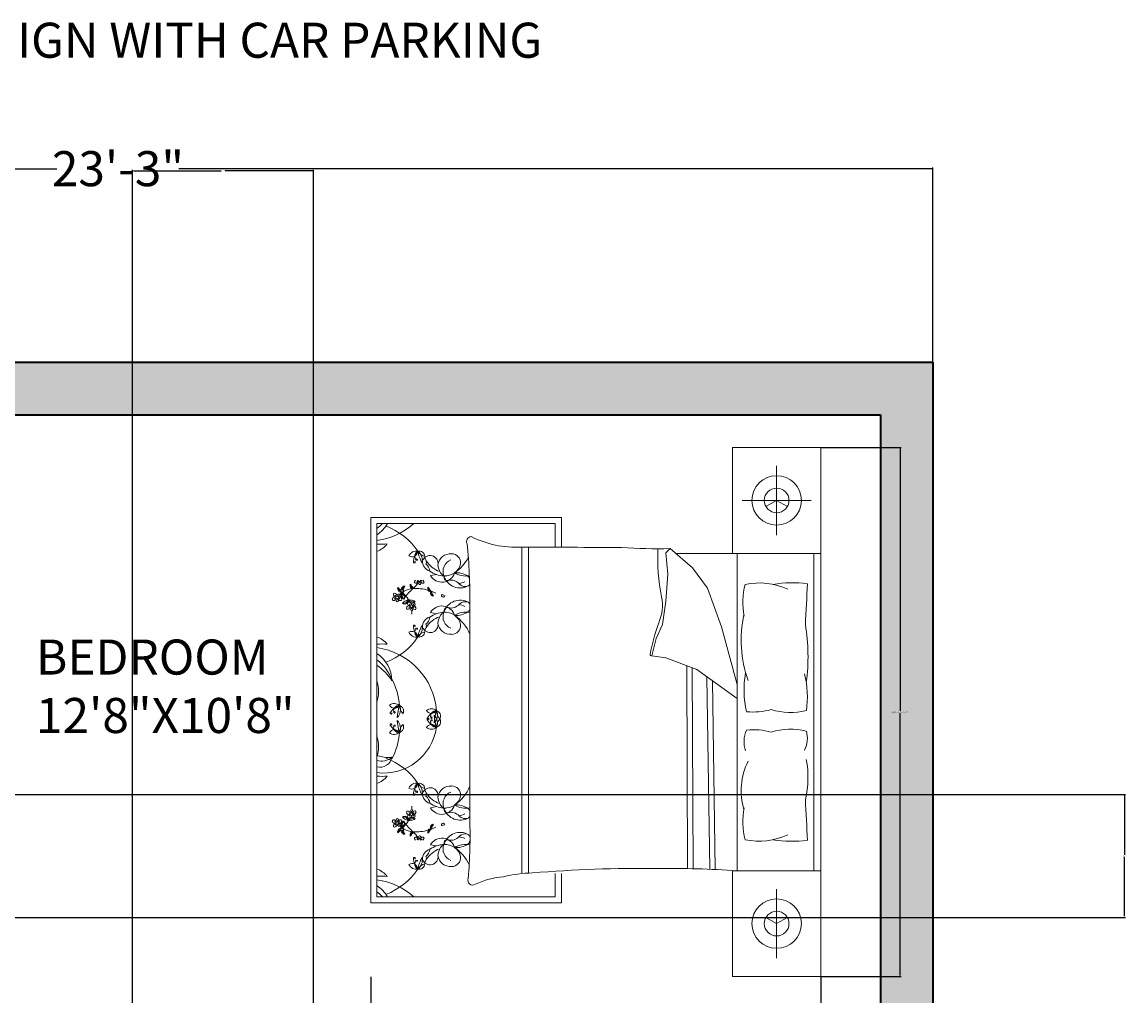
# Model space of a CAD drawing. Units: inches. Extents: x 37 to 706, y -568 to 110.
# Tile 24 of 24: x 517 to 706, y -57 to 110. Entities that reach past the tile are written whole.
import ezdxf

# ---------------------------------------------------------------- set-up
doc = ezdxf.new("R2010")
doc.units = ezdxf.units.IN
doc.header["$MEASUREMENT"] = 0
for name, color, linetype, lineweight in [('A-ANNO-DIMS', 2, 'Continuous', 18), ('A-ANNO-TEXT', 7, 'Continuous', 18), ('A-AREA-IDEN', 7, 'Continuous', 18), ('A-FURN', 8, 'Continuous', 13), ('A-WALL', 7, 'Continuous', 35), ('A-WALL-PATT', 252, 'Continuous', 13)]:
    doc.layers.add(name, color=color, linetype=linetype, lineweight=lineweight)
doc.styles.get("Standard").update_dxf_attribs({"font": 'arial.ttf'})
doc.dimstyles.get("Standard").update_dxf_attribs({"dimtxt": 0.18, "dimasz": 0.18, "dimexe": 0.18, "dimexo": 0.0625, "dimgap": 0.09, "dimtad": 0, "dimtih": 1, "dimtoh": 1, "dimdec": 0, "dimzin": 0, "dimdsep": 46, "dimlunit": 3, "dimtxsty": 'Standard', "dimcen": 0.09, "dimadec": 0, "dimazin": 0, "dimtfac": 1, "dimtdec": 0, "dimtofl": 0, "dimtmove": 0, "dimatfit": 3, "dimfxl": 1, "dimtolj": 1, "dimtzin": 0, "dimarcsym": 0})

# ---------------------------------------------------------------- blocks, each defined once
blk = doc.blocks.new('*D4')
at = {"layer": 'A-ANNO-DIMS', "color": 0, "lineweight": -2, "transparency": 16777216}
for p, q in [((393.96, 51.35), (393.96, 84.59)), ((394.14, 84.41), (523.01, 84.41)), ((672.78, 84.41), (543.91, 84.41)), ((672.96, 51.35), (672.96, 84.59))]:
    blk.add_line(p, q, dxfattribs=at)
at = {"layer": 'A-ANNO-DIMS', "color": 0, "transparency": 16777216}
for points in [[(394.14, 84.44), (394.14, 84.38), (393.96, 84.41)], [(672.78, 84.44), (672.78, 84.38), (672.96, 84.41)]]:
    blk.add_solid(points, dxfattribs=at)
at = {"layer": 'Defpoints', "color": 0, "transparency": 16777216}
for p in [(672.96, 84.41), (393.96, 51.29), (672.96, 51.29)]:
    blk.add_point(p, dxfattribs=at)
at = {"layer": 'A-ANNO-DIMS', "color": 0, "transparency": 16777216, "insert": (533.46, 84.41), "char_height": 6, "attachment_point": 5}
blk.add_mtext('\\A1;23\'-3"', dxfattribs=at)
blk = doc.blocks.new('BED-DOUBLE-WITH-NIGHTSTANDS')
for p, q in [((77.02, 90.57), (77.02, 0)), ((69.47, 75.59), (69.47, 87.43)), ((63.56, 81.51), (75.39, 81.51)), ((0, 78.61), (32.62, 78.61)), ((0, 12.59), (0, 78.61)), ((1.05, 77.56), (1.05, 13.64)), ((31.58, 77.56), (1.05, 77.56)), ((31.58, 73.49), (31.58, 77.56)), ((32.62, 78.61), (32.62, 73.49)), ((25.85, 17.62), (25.85, 73.5)), ((26.98, 17.7), (26.98, 73.5)), ((50.48, 72.53), (51.22, 73.26)), ((50.85, 68.86), (50.48, 72.53)), ((51.22, 73.26), (55.07, 69.96)), ((77.02, 72.45), (52.16, 72.45)), ((62.71, 72.45), (62.71, 18.11)), ((75.86, 18.11), (75.86, 72.45)), ((55.07, 69.96), (57.63, 66.48)), ((10.23, 68.64), (11.25, 68.84)), ((50.48, 64.28), (50.85, 68.86)), ((57.63, 66.48), (60.02, 59.87)), ((49.93, 60.24), (50.48, 64.28)), ((16.95, 26.9), (16.95, 63.67)), ((10.23, 62.31), (11.25, 62.11)), ((48.83, 57.86), (49.93, 60.24)), ((60.02, 59.87), (62.71, 50)), ((48.1, 54.92), (48.83, 57.86)), ((50.48, 54.55), (48.1, 54.92)), ((55.8, 52.54), (50.48, 54.55)), ((54.24, 18.43), (54.09, 53.18)), ((55.17, 18.44), (55.03, 52.83)), ((62.71, 47.57), (55.8, 52.54)), ((58.02, 18.39), (57.55, 51.28)), ((58.95, 18.36), (58.49, 50.6)), ((10.23, 28.89), (11.25, 29.09)), ((10.23, 22.56), (11.25, 22.36)), ((31.58, 13.64), (31.58, 17.63)), ((32.62, 17.61), (32.62, 12.59)), ((1.05, 13.64), (31.58, 13.64)), ((69.47, 14.97), (69.47, 3.14)), ((32.62, 12.59), (0, 12.59))]:
    blk.add_line(p, q)
for points in [[(61.93, 72.45), (61.93, 90.57), (77.02, 90.57)], [(69.47, 81.51), (67.64, 80.45)], [(69.47, 81.51), (71.3, 80.45)], [(77.02, 18.11), (61.93, 18.11), (61.93, 0), (77.02, 0)], [(69.47, 9.06), (67.64, 10.11)], [(69.47, 9.06), (71.3, 10.11)]]:
    blk.add_lwpolyline(points)
for points in [[(42.92, 73.45, 0.001242), (25.74, 73.5, -0.127202), (17.18, 75.31)], [(74.76, 67.25, 0.074897), (68.85, 67.14, -0.472817)], [(68.52, 45.71, 0.14099), (74.55, 45.53, 0.235245)], [(68.52, 41.84, -0.14099), (74.55, 42.02, -0.235245)], [(74.76, 23.32, -0.074897), (68.85, 23.42, 0.472817)], [(27.69, 17.73, 0.056112), (22.71, 17.07, 0.095341), (17.91, 15.8)]]:
    blk.add_lwpolyline(points, format="xyb")
for centre, radius in [((69.47, 81.51), 4.23), ((69.47, 81.51), 2.11), ((4.52, 64.91), 0.231), ((6.95, 63.41), 0.231), ((4.52, 26.28), 0.231), ((6.95, 27.79), 0.231), ((69.47, 9.06), 4.23), ((69.47, 9.06), 2.11)]:
    blk.add_circle(centre, radius)
for centre, radius, start, end in [((-3.2, 82.51), 7.18, 306.3036, 316.4814), ((-2.13, 80.43), 5.76, 303.4617, 330.1116), ((-0.54, 86.37), 11.83, 277.745, 311.8856), ((-1.71, 66.13), 11.83, 34.3865, 68.5908), ((-0.79, 77.21), 4.81, 292.5547, 318.9546), ((1.79, 90.38), 16.36, 267.4081, 273.6519), ((17.23, 74.48), 0.836, 93.98, 207.3412), ((-77.32, 64.75), 94.28, 359.3433, 5.6887), ((7.77, 71.53), 1.31, 77.7115, 159.0387), ((7.06, 72.84), 0.988, 238.4633, 358.2869), ((10.3, 70.85), 2.99, 138.8402, 177.9352), ((8.5, 71.96), 0.967, 117.6827, 223.7762), ((8.28, 71.86), 0.98, 2.9516, 103.728), ((16.12, 74.61), 8.27, 192.5173, 207.1824), ((6.95, 71.3), 1.87, 345.4653, 54.2343), ((9.77, 73.87), 2.02, 211.3827, 255.2969), ((10.16, 70.71), 1.36, 350.264, 160.8688), ((13.65, 70.21), 2.16, 84.9449, 172.8857), ((13.86, 70.84), 1.53, 354.4856, 91.0538), ((48.97, 156.3), 83.07, 265.8294, 271.553), ((83.29, 71.71), 34.18, 177.4519, 191.3392), ((7.46, 70.95), 0.147, 177.9352, 11.4834), ((7.53, 70.96), 0.0713, 11.4834, 127.9409), ((7.89, 71.38), 0.128, 223.7762, 159.7183), ((10.57, 71.04), 1.7, 175.969, 254.3045), ((8.69, 70.99), 0.833, 333.9755, 53.2681), ((8.31, 69.21), 1.81, 6.1662, 51.5825), ((13.15, 73.4), 4.28, 211.2614, 251.7045), ((14.13, 70.59), 2.63, 182.3591, 234.0401), ((14.47, 69.36), 2.1, 111.5819, 201.4221), ((12.73, 71.31), 2.72, 265.2933, 346.921), ((10.57, 74.83), 6.85, 303.6671, 333.2997), ((12.81, 73.44), 4.86, 236.2883, 266.5076), ((12.18, 69.76), 2.25, 209.9085, 343.1337), ((13.13, 68.34), 0.562, 167.3041, 285.1471), ((14.65, 65.65), 3.49, 122.7011, 126.3445), ((15.31, 69.41), 2.89, 199.2822, 299.1751), ((16.28, 72.32), 3.75, 238.8218, 279.1554), ((14.65, 65.65), 3.49, 55.785, 94.7304), ((15.95, 67.67), 1.09, 30.0293, 52.325), ((4.85, 66.4), 0.258, 124.3538, 214.3923), ((5.23, 66.36), 0.6, 190.3057, 287.1958), ((5.41, 66.58), 0.697, 176.9701, 248.2913), ((10.38, 70.25), 6.74, 212.6784, 216.3746), ((5.17, 66.41), 0.267, 216.3746, 291.7548), ((5.81, 66.23), 0.6, 122.8155, 187.3992), ((5.34, 65.98), 0.201, 289.3605, 111.7548), ((6.07, 66.15), 0.697, 109.4799, 177.6828), ((5.7, 66.59), 0.258, 56.8636, 146.9021), ((5.83, 66.31), 0.267, 148.8844, 224.2646), ((11.37, 62.96), 6.74, 145.1882, 148.8844), ((7.53, 62.67), 3.76, 94.756, 119.2041), ((15.54, 57.26), 12.37, 132.2412, 142.1744), ((9.29, 67.11), 2.55, 178.3264, 187.1302), ((6.53, 66.75), 0.476, 11.3256, 64.4621), ((8.15, 67.44), 1.43, 190.2588, 210.656), ((7.19, 66.85), 0.435, 188.3432, 274.2869), ((7.57, 67.09), 0.759, 210.656, 242.6341), ((8.14, 67.75), 1.46, 218.2101, 226.3071), ((7.07, 66.52), 0.185, 325.7657, 67.4417), ((1.34, 72.69), 8.6, 313.1541, 322.0459), ((7.72, 58.94), 7.5, 73.5842, 93.8277), ((7.66, 67.53), 0.177, 142.4737, 265.053), ((7.89, 67.56), 0.381, 127.7621, 169.0403), ((7.69, 67.89), 0.536, 265.053, 338.3618), ((8.4, 67.15), 0.7, 113.4276, 137.6104), ((8.32, 67.88), 0.231, 183.2768, 356.7232), ((8.49, 67.46), 0.377, 139.7889, 227.6792), ((8.37, 67.33), 0.199, 227.6792, 350.3487), ((7.6, 67.46), 0.755, 353.0852, 15.7171), ((8.1, 67.37), 0.477, 350.3487, 43.6538), ((8.98, 67.87), 0.555, 198.7263, 262.5032), ((8.54, 67.61), 0.22, 1.1081, 91.8675), ((8.68, 67.56), 0.385, 11.5637, 52.6358), ((8.95, 67.49), 0.178, 255.2356, 54.9248), ((12.34, 66.57), 2.55, 178.3264, 187.1302), ((9.58, 66.21), 0.476, 11.3256, 64.4621), ((11.19, 66.9), 1.43, 190.2588, 210.656), ((10.23, 66.31), 0.435, 188.3432, 274.2869), ((10.61, 66.55), 0.759, 210.656, 242.6341), ((11.19, 67.21), 1.46, 218.2101, 226.3071), ((10.11, 65.98), 0.185, 325.7657, 67.4417), ((13.76, 66), 1.86, 41.5653, 105.1471), ((14.78, 69.85), 2.6, 277.436, 299.9149), ((16.16, 68.13), 1.36, 221.5653, 293.8354), ((15.95, 67.67), 1.09, 314.4517, 333.558), ((75.82, 64.02), 12.14, 165.1039, 191.0369), ((66.47, 55.71), 11.67, 65.1316, 101.7583), ((936.66, 17.33), 863.34, 176.68521, 177.14978), ((3.86, 64.56), 0.177, 142.4737, 265.053), ((4.09, 64.6), 0.381, 61.2196, 169.0403), ((3.89, 64.92), 0.536, 265.053, 338.3618), ((4.34, 65.38), 0.455, 157.4086, 261.4386), ((4.09, 65.4), 0.229, 58.0499, 135.6268), ((4.6, 64.19), 0.7, 113.4276, 137.6104), ((4.32, 65.26), 0.153, 172.906, 277.132), ((3.82, 64.98), 0.727, 14.7558, 58.0499), ((4.69, 64.5), 0.377, 139.7889, 227.6792), ((4.57, 64.37), 0.199, 227.6792, 350.3487), ((4.84, 65.17), 0.315, 36.1046, 181.4281), ((3.8, 64.5), 0.755, 353.0852, 15.7171), ((4.29, 64.41), 0.477, 350.3487, 43.6538), ((5.18, 64.9), 0.555, 198.7263, 262.5032), ((4.66, 65.42), 0.317, 270.0645, 331.1507), ((4.93, 65.34), 0.363, 221.8413, 265.7877), ((4.74, 64.65), 0.22, 1.1081, 91.8675), ((4.92, 65.2), 0.226, 263.7526, 41.7054), ((4.88, 64.6), 0.385, 11.5637, 86.365), ((7.53, 62.67), 3.76, 124.0033, 132.4917), ((5.15, 64.53), 0.178, 255.2356, 54.9248), ((3.66, 62.2), 4.02, 63.7819, 68.2913), ((5.81, 65.29), 0.639, 128.3208, 208.8162), ((5.92, 65.34), 0.764, 207.7043, 254.3516), ((5.49, 65.98), 0.201, 221.8703, 44.2646), ((6.41, 65.39), 1.05, 157.2305, 229.0635), ((6.05, 65.74), 0.619, 174.4544, 220.6188), ((5.43, 64.9), 1.05, 270.278, 342.111), ((6.13, 63.58), 0.744, 98.7227, 159.3375), ((2.53, 62.29), 4.51, 30.544, 49.818), ((5.02, 64.86), 0.744, 340.0041, 40.6188), ((5.92, 64.93), 0.619, 278.7227, 324.8872), ((5.81, 64.43), 0.639, 290.5253, 358.5375), ((7.06, 64.61), 0.639, 182.8499, 266.1226), ((6.81, 65.06), 0.619, 231.7607, 277.9252), ((7.29, 65.17), 1.05, 214.5369, 286.3699), ((7, 63.71), 0.744, 37.3105, 97.9252), ((10.63, 65.65), 0.435, 147.5332, 233.4768), ((11.02, 65.87), 0.759, 179.1859, 211.164), ((10.28, 65.7), 0.185, 354.3784, 96.0543), ((7.72, 58.94), 7.5, 63.0032, 69.8941), ((11.6, 66.22), 1.43, 211.164, 231.5612), ((11.85, 67.38), 2.55, 234.6898, 243.4936), ((11.87, 66.07), 1.46, 195.5129, 203.6099), ((10.23, 65.12), 0.476, 357.3579, 50.4944), ((12.28, 65.21), 0.175, 12.7051, 190.4384), ((12.38, 65.23), 0.284, 190.4384, 10.4136), ((15.31, 61.54), 2.89, 60.8249, 160.7178), ((42.55, 63.54), 7.37, 336.2616, 11.3392), ((5.75, 64.54), 0.764, 244.9899, 291.6373), ((6.29, 63.06), 0.177, 142.4737, 265.053), ((6.52, 63.09), 0.381, 61.2196, 169.0403), ((6.32, 63.41), 0.536, 265.053, 338.3618), ((6.77, 63.88), 0.455, 157.4086, 261.4386), ((6.52, 63.89), 0.229, 58.0499, 135.6268), ((7.03, 62.68), 0.7, 113.4276, 137.6104), ((6.76, 63.75), 0.153, 172.906, 277.132), ((6.25, 63.47), 0.727, 14.7558, 58.0499), ((2.53, 62.29), 4.51, 23.0501, 23.8477), ((7.12, 62.99), 0.377, 139.7889, 227.6792), ((7, 62.86), 0.199, 227.6792, 350.3487), ((7.27, 63.66), 0.315, 36.1046, 181.4281), ((6.23, 62.99), 0.755, 353.0852, 15.7171), ((7.08, 64.73), 0.764, 265.0106, 311.658), ((2.53, 62.29), 4.51, 357.1071, 4.7585), ((6.72, 62.9), 0.477, 350.3487, 43.6538), ((7.61, 63.4), 0.555, 198.7263, 262.5032), ((7.09, 63.91), 0.317, 270.0645, 331.1507), ((7.36, 63.83), 0.363, 221.8413, 265.7877), ((7.17, 63.14), 0.22, 1.1081, 91.8675), ((7.36, 63.7), 0.226, 263.7526, 41.7054), ((7.31, 63.09), 0.385, 11.5637, 86.365), ((7.58, 63.02), 0.178, 255.2356, 54.9248), ((12.81, 57.5), 4.86, 93.4924, 123.7117), ((12.18, 61.19), 2.25, 16.8663, 150.0915), ((14.13, 60.36), 2.63, 125.9599, 177.6409), ((14.47, 61.59), 2.1, 158.5779, 248.4181), ((12.73, 59.64), 2.72, 13.079, 94.7067), ((13.13, 62.61), 0.562, 74.8529, 192.6959), ((14.65, 65.3), 3.49, 233.6555, 237.2989), ((13.76, 64.95), 1.86, 254.8529, 318.4347), ((16.28, 58.63), 3.75, 79.7133, 121.1782), ((14.65, 65.3), 3.49, 265.2696, 304.215), ((14.78, 61.1), 2.6, 60.0851, 82.564), ((16.16, 62.82), 1.36, 66.1646, 138.4347), ((15.95, 63.28), 1.09, 307.675, 336.7144), ((15.95, 63.28), 1.09, 23.229, 45.5483), ((10.57, 59.91), 1.7, 105.6955, 184.031), ((10.16, 60.24), 1.36, 199.1312, 9.736), ((8.31, 61.74), 1.81, 308.4175, 353.8338), ((13.15, 57.54), 4.28, 108.2955, 148.7386), ((13.65, 60.74), 2.16, 187.1143, 275.0551), ((10.57, 56.11), 6.85, 21.4941, 56.3329), ((82.33, 48.63), 35.12, 160.1194, 169.3383), ((84.45, 57.63), 21.05, 168.0397, 199.2615), ((7.06, 58.1), 0.988, 1.7131, 121.5367), ((7.77, 59.41), 1.31, 200.9613, 282.2885), ((7.46, 60), 0.147, 348.5166, 182.0648), ((10.3, 60.1), 2.99, 182.0648, 221.1598), ((7.53, 59.98), 0.0713, 232.0591, 348.5166), ((8.5, 58.99), 0.967, 136.2238, 242.3173), ((7.94, 59.56), 0.0771, 200.2667, 136.2271), ((6.95, 59.65), 1.87, 305.7657, 14.5347), ((16.12, 56.34), 8.27, 152.8176, 167.4827), ((8.28, 59.09), 0.98, 256.272, 357.0484), ((9.77, 57.08), 2.02, 104.7031, 148.6173), ((8.69, 59.96), 0.833, 306.7319, 26.0245), ((13.86, 60.11), 1.53, 268.9462, 5.5144), ((41.99, 54.84), 32.85, 352.2196, 9.497), ((-0.79, 53.74), 4.81, 41.0454, 67.4453), ((1.79, 40.57), 16.36, 86.3481, 92.5919), ((-1.71, 64.81), 11.83, 291.4092, 325.6135), ((-0.54, 44.58), 11.83, 4.4623, 82.255), ((-2.13, 50.51), 5.76, 1.272, 56.5383), ((48.03, 55.13), 0.219, 178.8623, 289.7536), ((-3.2, 48.44), 7.18, 17.8504, 53.6964), ((-5.22, 44.66), 10.68, 34.0123, 54.053), ((79.85, 49.11), 15.97, 169.8617, 193.6238), ((58.59, 47.9), 16.14, 351.5249, 13.96), ((-5.17, 48.79), 6.5, 343.5431, 17.0202), ((-6.88, 45.48), 11.83, 4.4623, 27.4146), ((-8.52, 46.22), 9.62, 4.3787, 5.6357), ((-15.11, 41.15), 17.18, 19.7217, 19.9028), ((4.03, 45.43), 1.31, 47.7873, 129.1145), ((4.07, 46.92), 0.988, 208.5391, 328.3627), ((5.88, 43.58), 2.99, 108.9159, 148.011), ((4.87, 45.44), 0.967, 87.7585, 193.852), ((4.06, 45.24), 0.128, 193.852, 129.9245), ((12.81, 43.93), 8.27, 162.593, 177.2582), ((3.21, 45.64), 1.87, 315.5411, 24.3101), ((6.93, 46.46), 2.02, 181.4585, 225.3727), ((4.64, 45.46), 0.98, 333.0274, 73.8037), ((10.37, 44.53), 1.31, 47.7873, 129.1145), ((10.41, 46.02), 0.988, 208.5391, 328.3627), ((12.22, 42.67), 2.99, 108.9159, 148.011), ((11.21, 44.53), 0.967, 87.7585, 193.852), ((9.54, 44.73), 1.87, 315.5411, 24.3101), ((19.14, 43.02), 8.27, 162.593, 177.2582), ((10.97, 44.56), 0.98, 333.0274, 73.8037), ((13.27, 45.55), 2.02, 181.4585, 225.3727), ((65.49, 56.38), 11.1, 264.0129, 285.8293), ((3.47, 45.08), 0.147, 148.011, 341.5592), ((3.54, 45.06), 0.0713, 341.5592, 98.0167), ((12.81, 44.25), 8.27, 182.7418, 197.407), ((3.21, 42.54), 1.87, 335.6899, 44.4589), ((9.8, 44.18), 0.147, 148.011, 341.5592), ((9.8, 44), 0.147, 18.4408, 211.989), ((12.22, 45.51), 2.99, 211.989, 251.0841), ((9.88, 44.15), 0.0713, 341.5592, 98.0167), ((9.88, 44.03), 0.0713, 261.9833, 18.4408), ((11.21, 43.65), 0.967, 166.148, 272.2415), ((10.39, 44.33), 0.128, 193.852, 129.9245), ((10.44, 43.86), 0.0771, 230.1909, 166.0209), ((9.54, 43.45), 1.87, 335.6899, 44.4589), ((19.14, 45.16), 8.27, 182.7418, 197.407), ((10.97, 43.62), 0.98, 286.1963, 26.9726), ((13.27, 42.63), 2.02, 134.6273, 178.5415), ((2.19, 43.98), 9.15, 262.8636, 351.8197), ((4.07, 41.26), 0.988, 31.6373, 151.4609), ((4.03, 42.75), 1.31, 230.8855, 312.2127), ((3.47, 43.1), 0.147, 18.4408, 211.989), ((5.88, 44.6), 2.99, 211.989, 251.0841), ((3.54, 43.12), 0.0713, 261.9833, 18.4408), ((-6.88, 42.69), 11.83, 332.5854, 355.5377), ((4.87, 42.74), 0.967, 166.148, 272.2415), ((4.11, 42.95), 0.0771, 230.1909, 166.0209), ((6.93, 41.72), 2.02, 134.6273, 178.5415), ((4.64, 42.72), 0.98, 286.1963, 26.9726), ((10.41, 42.16), 0.988, 31.6373, 151.4609), ((10.37, 43.65), 1.31, 230.8855, 312.2127), ((68.68, 40.17), 4.8, 155.0183, 198.5407), ((65.49, 31.16), 11.1, 74.1707, 95.9871), ((70.25, 40.78), 4.48, 333.3437, 16.1026), ((-5.17, 39.39), 6.5, 342.9798, 16.4569), ((-8.52, 41.96), 9.62, 354.3643, 355.6213), ((-15.11, 47.03), 17.18, 340.0972, 340.2783), ((3.02, 42.8), 5.3, 248.117, 276.6195), ((1.55, 37.94), 2.12, 256.3898, 349.0739), ((1.84, 39.54), 2.68, 252.8609, 311.9049), ((-1.71, 26.39), 11.83, 34.3865, 68.5908), ((74.93, 31.78), 11.53, 153.8761, 196.1746), ((58.92, 34.06), 15.92, 346.3427, 11.1841), ((1.79, 50.63), 16.36, 267.4081, 273.6519), ((-0.79, 37.46), 4.81, 292.5547, 318.9546), ((7.77, 31.78), 1.31, 77.7115, 159.0387), ((7.06, 33.09), 0.988, 238.4633, 358.2869), ((10.3, 31.1), 2.99, 138.8402, 177.9352), ((8.5, 32.21), 0.967, 117.6827, 223.7762), ((8.28, 32.11), 0.98, 2.9516, 103.728), ((9.77, 34.12), 2.02, 211.3827, 255.2969), ((6.95, 31.55), 1.87, 345.4653, 54.2343), ((16.12, 34.86), 8.27, 192.5173, 207.1824), ((10.16, 30.96), 1.36, 350.264, 160.8688), ((13.65, 30.46), 2.16, 84.9449, 172.8857), ((13.86, 31.09), 1.53, 354.4856, 91.0538), ((10.57, 35.08), 6.85, 303.6671, 338.5059), ((7.46, 31.2), 0.147, 177.9352, 11.4834), ((7.53, 31.21), 0.0713, 11.4834, 127.9409), ((7.89, 31.63), 0.128, 223.7762, 159.7183), ((10.57, 31.29), 1.7, 175.969, 254.3045), ((8.69, 31.24), 0.833, 333.9755, 53.2681), ((8.31, 29.46), 1.81, 6.1662, 51.5825), ((13.15, 33.66), 4.28, 211.2614, 251.7045), ((14.13, 30.84), 2.63, 182.3591, 234.0401), ((14.47, 29.61), 2.1, 111.5819, 201.4221), ((12.73, 31.56), 2.72, 265.2933, 346.921), ((936.66, 73.23), 863.34, 182.85022, 183.31479), ((7.12, 28.21), 0.377, 132.3208, 220.2111), ((7, 28.34), 0.199, 9.6513, 132.3208), ((2.53, 28.91), 4.51, 355.2415, 2.8929), ((6.72, 28.3), 0.477, 316.3462, 9.6513), ((7.61, 27.8), 0.555, 97.4968, 161.2737), ((7.58, 28.18), 0.178, 305.0752, 104.7644), ((12.81, 33.7), 4.86, 236.2883, 266.5076), ((12.18, 30.01), 2.25, 209.9085, 343.1337), ((13.13, 28.59), 0.562, 167.3041, 285.1471), ((14.65, 25.9), 3.49, 122.7011, 126.3445), ((15.31, 29.66), 2.89, 199.2822, 299.1751), ((16.28, 32.57), 3.75, 238.8218, 280.2867), ((14.65, 25.9), 3.49, 55.785, 94.7304), ((15.95, 27.92), 1.09, 23.2856, 52.325), ((75.82, 26.55), 12.14, 168.9631, 194.8961), ((3.86, 26.63), 0.177, 94.947, 217.5263), ((4.09, 26.6), 0.381, 190.9597, 298.7804), ((3.89, 26.28), 0.536, 21.6382, 94.947), ((4.6, 27.01), 0.7, 222.3896, 246.5724), ((4.69, 26.7), 0.377, 132.3208, 220.2111), ((4.57, 26.83), 0.199, 9.6513, 132.3208), ((3.8, 26.7), 0.755, 344.2829, 6.9148), ((4.29, 26.79), 0.477, 316.3462, 9.6513), ((5.18, 26.29), 0.555, 97.4968, 161.2737), ((4.74, 26.55), 0.22, 268.1325, 358.8919), ((4.88, 26.6), 0.385, 273.635, 348.4363), ((5.15, 26.67), 0.178, 305.0752, 104.7644), ((5.92, 25.86), 0.764, 105.6484, 152.2957), ((6.41, 25.8), 1.05, 130.9365, 202.7695), ((5.75, 26.66), 0.764, 68.3627, 115.0101), ((5.43, 26.3), 1.05, 17.889, 89.722), ((6.13, 27.61), 0.744, 200.6625, 261.2773), ((2.53, 28.91), 4.51, 310.182, 329.456), ((5.02, 26.34), 0.744, 319.3812, 19.9959), ((5.92, 26.27), 0.619, 35.1128, 81.2773), ((5.81, 26.77), 0.639, 1.4625, 69.4747), ((6.29, 28.14), 0.177, 94.947, 217.5263), ((6.52, 28.11), 0.381, 190.9597, 298.7804), ((6.32, 27.78), 0.536, 21.6382, 94.947), ((6.77, 27.32), 0.455, 98.5614, 202.5914), ((6.52, 27.31), 0.229, 224.3732, 301.9501), ((7.06, 26.59), 0.639, 93.8774, 177.1501), ((7.29, 26.03), 1.05, 73.6301, 145.4631), ((6.81, 26.14), 0.619, 82.0748, 128.2393), ((7.03, 28.52), 0.7, 222.3896, 246.5724), ((6.76, 27.45), 0.153, 82.868, 187.094), ((6.25, 27.73), 0.727, 301.9501, 345.2442), ((2.53, 28.91), 4.51, 336.1523, 336.9499), ((7, 27.49), 0.744, 262.0748, 322.6895), ((6.23, 28.2), 0.755, 344.2829, 6.9148), ((7.27, 27.54), 0.315, 178.5719, 323.8954), ((7.08, 26.46), 0.764, 48.342, 94.9894), ((7.36, 27.37), 0.363, 94.2123, 138.1587), ((7.09, 27.29), 0.317, 28.8493, 89.9355), ((7.17, 28.06), 0.22, 268.1325, 358.8919), ((7.31, 28.11), 0.385, 273.635, 348.4363), ((7.36, 27.5), 0.226, 318.2946, 96.2474), ((13.76, 26.25), 1.86, 41.5653, 105.1471), ((14.78, 30.1), 2.6, 277.436, 299.9149), ((16.16, 28.38), 1.36, 221.5653, 293.8354), ((-71.13, 24.12), 88.13, 355.2402, 1.8035), ((15.95, 27.92), 1.09, 314.4517, 336.7144), ((4.34, 25.81), 0.455, 98.5614, 202.5914), ((4.09, 25.8), 0.229, 224.3732, 301.9501), ((4.32, 25.94), 0.153, 82.868, 187.094), ((3.82, 26.22), 0.727, 301.9501, 345.2442), ((4.84, 26.03), 0.315, 178.5719, 323.8954), ((4.85, 24.8), 0.258, 145.6077, 235.6462), ((5.23, 24.83), 0.6, 72.8042, 169.6943), ((4.93, 25.86), 0.363, 94.2123, 138.1587), ((4.66, 25.78), 0.317, 28.8493, 89.9355), ((5.41, 24.62), 0.697, 111.7087, 183.0299), ((10.38, 20.95), 6.74, 143.6254, 147.3216), ((4.92, 25.99), 0.226, 318.2946, 96.2474), ((5.17, 24.78), 0.267, 68.2452, 143.6254), ((7.53, 28.53), 3.76, 227.5083, 235.9967), ((3.66, 29), 4.02, 291.7087, 296.2181), ((5.81, 25.91), 0.639, 151.1838, 231.6792), ((5.81, 24.97), 0.6, 172.6008, 237.1845), ((5.34, 25.22), 0.201, 248.2452, 70.6395), ((5.49, 25.22), 0.201, 315.7354, 138.1297), ((6.07, 25.05), 0.697, 182.3172, 250.5201), ((6.05, 25.46), 0.619, 139.3812, 185.5456), ((5.83, 24.89), 0.267, 135.7354, 211.1156), ((11.37, 28.24), 6.74, 211.1156, 214.8118), ((7.53, 28.53), 3.76, 240.7959, 265.244), ((15.54, 33.94), 12.37, 217.8256, 227.7588), ((7.19, 24.34), 0.435, 85.7131, 171.6568), ((7.57, 24.1), 0.759, 117.3659, 149.344), ((7.07, 24.67), 0.185, 292.5583, 34.2343), ((7.72, 32.26), 7.5, 266.1723, 286.4158), ((1.34, 18.5), 8.6, 37.9541, 46.8459), ((11.19, 24.3), 1.43, 149.344, 169.7412), ((12.34, 24.63), 2.55, 172.8698, 181.6736), ((9.58, 24.98), 0.476, 295.5379, 348.6744), ((10.23, 24.88), 0.435, 85.7131, 171.6568), ((10.61, 24.64), 0.759, 117.3659, 149.344), ((11.19, 23.99), 1.46, 133.6929, 141.7899), ((10.11, 25.21), 0.185, 292.5583, 34.2343), ((10.63, 25.55), 0.435, 126.5232, 212.4668), ((11.02, 25.33), 0.759, 148.836, 180.8141), ((10.28, 25.5), 0.185, 263.9457, 5.6216), ((7.72, 32.26), 7.5, 290.1059, 296.9968), ((11.6, 24.98), 1.43, 128.4388, 148.836), ((11.85, 23.82), 2.55, 116.5064, 125.3102), ((11.87, 25.13), 1.46, 156.3901, 164.4871), ((10.23, 26.08), 0.476, 309.5056, 2.6421), ((12.28, 25.98), 0.175, 169.5616, 347.2949), ((12.38, 25.96), 0.284, 349.5864, 169.5616), ((15.31, 21.79), 2.89, 60.8249, 160.7178), ((5.7, 24.61), 0.258, 213.0979, 303.1364), ((8.15, 23.76), 1.43, 149.344, 169.7412), ((9.29, 24.09), 2.55, 172.8698, 181.6736), ((6.53, 24.45), 0.476, 295.5379, 348.6744), ((8.14, 23.45), 1.46, 133.6929, 141.7899), ((7.66, 23.67), 0.177, 94.947, 217.5263), ((7.89, 23.64), 0.381, 190.9597, 232.2379), ((7.69, 23.31), 0.536, 21.6382, 94.947), ((8.4, 24.05), 0.7, 222.3896, 246.5724), ((8.32, 23.32), 0.231, 3.2768, 176.7232), ((8.49, 23.74), 0.377, 132.3208, 220.2111), ((8.37, 23.87), 0.199, 9.6513, 132.3208), ((7.6, 23.73), 0.755, 344.2829, 6.9148), ((8.1, 23.82), 0.477, 316.3462, 9.6513), ((8.98, 23.33), 0.555, 97.4968, 161.2737), ((8.54, 23.59), 0.22, 268.1325, 358.8919), ((8.95, 23.71), 0.178, 305.0752, 104.7644), ((8.68, 23.64), 0.385, 307.3642, 348.4363), ((12.18, 21.44), 2.25, 16.8663, 150.0915), ((14.13, 20.61), 2.63, 125.9599, 177.6409), ((13.13, 22.86), 0.562, 74.8529, 192.6959), ((14.65, 25.55), 3.49, 233.6555, 237.2989), ((13.76, 25.2), 1.86, 254.8529, 318.4347), ((14.78, 21.35), 2.6, 60.0851, 82.564), ((16.16, 23.07), 1.36, 66.1646, 138.4347), ((15.95, 23.53), 1.09, 307.675, 342.5814), ((15.95, 23.53), 1.09, 16.6343, 45.5483), ((66.47, 34.85), 11.67, 258.2417, 294.8684), ((10.57, 20.16), 1.7, 105.6955, 184.031), ((8.31, 21.99), 1.81, 308.4175, 353.8338), ((13.15, 17.79), 4.28, 108.2955, 148.7386), ((12.81, 17.75), 4.86, 93.4924, 123.7117), ((14.47, 21.84), 2.1, 158.5779, 248.4181), ((12.73, 19.89), 2.72, 13.079, 94.7067), ((16.28, 18.88), 3.75, 79.249, 121.1782), ((14.65, 25.55), 3.49, 265.2696, 304.215), ((10.57, 16.37), 6.85, 23.6453, 56.3329), ((7.06, 18.36), 0.988, 1.7131, 121.5367), ((7.77, 19.67), 1.31, 200.9613, 282.2885), ((7.46, 20.25), 0.147, 348.5166, 182.0648), ((10.3, 20.35), 2.99, 182.0648, 221.1598), ((7.53, 20.24), 0.0713, 232.0591, 348.5166), ((8.5, 19.24), 0.967, 136.2238, 242.3173), ((7.94, 19.81), 0.0771, 200.2667, 136.2271), ((16.12, 16.59), 8.27, 152.8176, 167.4827), ((6.95, 19.9), 1.87, 305.7657, 14.5347), ((9.77, 17.33), 2.02, 104.7031, 148.6173), ((8.28, 19.34), 0.98, 256.272, 357.0484), ((10.16, 20.49), 1.36, 199.1312, 9.736), ((8.69, 20.21), 0.833, 306.7319, 26.0245), ((13.65, 20.99), 2.16, 187.1143, 275.0551), ((13.86, 20.36), 1.53, 268.9462, 5.5144), ((-0.79, 13.99), 4.81, 41.0454, 67.4453), ((1.79, 0.82), 16.36, 86.3481, 92.5919), ((-1.71, 25.06), 11.83, 291.4092, 325.6135), ((45.72, -193.78), 212.28, 89.1145, 94.8735), ((51.64, -144.24), 162.73, 86.1, 90.9282), ((-0.54, 4.83), 11.83, 48.1144, 82.255), ((-2.13, 10.76), 5.76, 29.8884, 56.5383), ((17.45, 16.48), 0.826, 156.5219, 303.8264), ((-3.2, 8.69), 7.18, 43.5186, 53.6964)]:
    blk.add_arc(centre, radius, start, end)
blk = doc.blocks.new('*D23')
at = {"layer": 'A-ANNO-DIMS', "color": 0, "lineweight": -2, "transparency": 16777216}
for p, q in [((653.81, 36.66), (667.51, 36.66)), ((667.33, 36.48), (667.33, -8.44)), ((667.33, -53.72), (667.33, -8.8)), ((653.81, -53.9), (667.51, -53.9))]:
    blk.add_line(p, q, dxfattribs=at)
at = {"layer": 'A-ANNO-DIMS', "color": 0, "transparency": 16777216}
for points in [[(667.3, 36.48), (667.36, 36.48), (667.33, 36.66)], [(667.3, -53.72), (667.36, -53.72), (667.33, -53.9)]]:
    blk.add_solid(points, dxfattribs=at)
at = {"layer": 'Defpoints', "color": 0, "transparency": 16777216}
for p in [(653.75, 36.66), (667.33, 36.66), (653.75, -53.9)]:
    blk.add_point(p, dxfattribs=at)
at = {"layer": 'A-ANNO-DIMS', "color": 0, "transparency": 16777216, "insert": (667.33, -8.62), "char_height": 0.18, "attachment_point": 5}
blk.add_mtext('\\A1;BED GROUP 7\'-6 1/2" TYP.', dxfattribs=at)
blk = doc.blocks.new('*D24')
at = {"layer": 'A-ANNO-DIMS', "color": 0, "lineweight": -2, "transparency": 16777216}
for p, q in [((576.73, -53.97), (576.73, -67.67)), ((653.75, -53.97), (653.75, -67.67)), ((576.91, -67.49), (614.6, -67.49)), ((653.57, -67.49), (615.88, -67.49))]:
    blk.add_line(p, q, dxfattribs=at)
at = {"layer": 'A-ANNO-DIMS', "color": 0, "transparency": 16777216}
for points in [[(576.91, -67.46), (576.91, -67.52), (576.73, -67.49)], [(653.57, -67.46), (653.57, -67.52), (653.75, -67.49)]]:
    blk.add_solid(points, dxfattribs=at)
at = {"layer": 'Defpoints', "color": 0, "transparency": 16777216}
for p in [(576.73, -53.9), (653.75, -53.9), (653.75, -67.49)]:
    blk.add_point(p, dxfattribs=at)
at = {"layer": 'A-ANNO-DIMS', "color": 0, "transparency": 16777216, "insert": (615.24, -67.49), "char_height": 0.18, "attachment_point": 5}
blk.add_mtext('\\A1;6\'-5" TYP.', dxfattribs=at)
blk = doc.blocks.new('*D52')
at = {"layer": 'A-ANNO-DIMS', "color": 0, "lineweight": -2, "transparency": 16777216}
for p, q in [((535.96, -303.65), (535.96, 84.22)), ((536.14, 84.04), (551.13, 84.04)), ((566.78, 84.04), (551.79, 84.04)), ((566.96, -303.65), (566.96, 84.22))]:
    blk.add_line(p, q, dxfattribs=at)
at = {"layer": 'A-ANNO-DIMS', "color": 0, "transparency": 16777216}
for points in [[(536.14, 84.07), (536.14, 84.01), (535.96, 84.04)], [(566.78, 84.07), (566.78, 84.01), (566.96, 84.04)]]:
    blk.add_solid(points, dxfattribs=at)
at = {"layer": 'Defpoints', "color": 0, "transparency": 16777216}
for p in [(566.96, 84.04), (535.96, -303.71), (566.96, -303.71)]:
    blk.add_point(p, dxfattribs=at)
at = {"layer": 'A-ANNO-DIMS', "color": 0, "transparency": 16777216, "insert": (551.46, 84.04), "char_height": 0.18, "attachment_point": 5}
blk.add_mtext('\\A1;2\'-7"', dxfattribs=at)
blk = doc.blocks.new('*D57')
at = {"layer": 'A-ANNO-DIMS', "color": 0, "lineweight": -2, "transparency": 16777216}
for p, q in [((473.38, -22.71), (705.89, -22.71)), ((705.71, -22.89), (705.71, -33.06)), ((705.71, -43.59), (705.71, -33.42)), ((473.38, -43.77), (705.89, -43.77))]:
    blk.add_line(p, q, dxfattribs=at)
at = {"layer": 'A-ANNO-DIMS', "color": 0, "transparency": 16777216}
for points in [[(705.68, -22.89), (705.74, -22.89), (705.71, -22.71)], [(705.68, -43.59), (705.74, -43.59), (705.71, -43.77)]]:
    blk.add_solid(points, dxfattribs=at)
at = {"layer": 'Defpoints', "color": 0, "transparency": 16777216}
for p in [(473.32, -22.71), (473.32, -43.77), (705.71, -43.77)]:
    blk.add_point(p, dxfattribs=at)
at = {"layer": 'A-ANNO-DIMS', "color": 0, "transparency": 16777216, "insert": (705.71, -33.24), "char_height": 0.18, "attachment_point": 5}
blk.add_mtext('\\A1;1\'-9"', dxfattribs=at)

msp = doc.modelspace()

# ---------------------------------------------------------------- hatches: boundary and pattern name
at = {"layer": 'A-WALL-PATT'}
h = msp.add_hatch(color=256, dxfattribs=at)
h.dxf.hatch_style = 1
h.paths.add_polyline_path([(220.96, -351.71), (211.96, -351.71), (211.96, -513.71), (254.96, -513.71), (254.96, -504.71), (220.96, -504.71)], flags=17)
h.paths.add_polyline_path([(220.96, -294.71), (211.96, -294.71), (211.96, -303.71), (220.96, -303.71)], flags=17)
h.paths.add_polyline_path([(175.96, -294.71), (155.87, -294.71), (155.87, -303.71), (155.96, -303.71), (175.96, -303.71)], flags=17)
h.paths.add_polyline_path([(220.96, -16.71), (211.96, -16.71), (211.96, -142.71), (220.96, -142.71)], flags=17)
h.paths.add_polyline_path([(357.96, 51.29), (78.96, 51.29), (78.96, -513.71), (87.96, -513.71), (87.96, -303.71), (95.87, -303.71), (95.87, -294.71), (87.96, -294.71), (87.96, -142.71), (187.96, -142.71), (187.96, -133.71), (87.96, -133.71), (87.96, -25.71), (106.96, -25.71), (106.96, -16.71), (87.96, -16.71), (87.96, 42.29), (348.96, 42.29), (348.96, 17.13), (348.96, -133.71), (246.96, -133.71), (246.96, -142.71), (348.96, -142.71), (348.96, -294.71), (251.96, -294.71), (251.96, -303.71), (348.96, -303.71), (348.96, -351.71), (260.96, -351.71), (260.96, -329.71), (251.96, -329.71), (251.96, -360.71), (327.45, -360.71), (348.96, -360.71), (348.96, -504.71), (314.96, -504.71), (314.96, -513.71), (357.96, -513.71)])
h.paths.add_polyline_path([(416.96, -303.71), (402.96, -303.71), (402.96, -151.71), (478.96, -151.71), (478.96, -142.71), (402.96, -142.71), (402.96, -22.71), (409.96, -22.71), (409.96, -13.71), (402.96, -13.71), (402.96, 42.29), (663.96, 42.29), (663.96, -303.71), (566.96, -303.71), (566.96, -312.71), (663.96, -312.71), (663.96, -360.71), (575.96, -360.71), (575.96, -338.71), (566.96, -338.71), (566.96, -360.71), (566.96, -369.71), (642.45, -369.71), (663.96, -369.71), (663.96, -513.71), (629.96, -513.71), (629.96, -522.71), (672.96, -522.71), (672.96, 51.29), (393.96, 51.29), (393.96, -522.71), (402.96, -522.71), (402.96, -312.71), (416.96, -312.71)])
h.paths.add_polyline_path([(490.96, -303.71), (476.96, -303.71), (476.96, -312.71), (490.96, -312.71)], flags=17)
h.paths.add_polyline_path([(535.96, -303.71), (526.96, -303.71), (526.96, -312.71), (535.96, -312.71)], flags=17)
h.paths.add_polyline_path([(535.96, -369.71), (526.96, -369.71), (526.96, -522.71), (569.96, -522.71), (569.96, -513.71), (535.96, -513.71)], flags=17)
h.paths.add_polyline_path([(511.96, -13.71), (502.96, -13.71), (502.96, -151.71), (511.96, -151.71)], flags=17)
h.paths.add_polyline_path([(651.54, -142.71), (651.54, -120.18), (642.54, -120.18), (642.54, -142.71), (550.54, -142.71), (550.54, -120.71), (541.54, -120.71), (541.54, -142.71), (537.96, -142.71), (537.96, -151.71), (651.54, -151.71)], flags=17)
h.paths.add_polyline_path([(651.54, -85.71), (541.54, -85.71), (541.54, -94.71), (651.54, -94.71)], flags=17)
h.paths.add_polyline_path([(476.96, -13.71), (469.96, -13.71), (469.96, -22.71), (476.96, -22.71)], flags=17)
h.paths.add_polyline_path([(185.96, -16.71), (166.96, -16.71), (166.96, -25.71), (185.96, -25.71)], flags=17)
h.paths.add_polyline_path([(168.91, -414.72), (214.62, -414.72), (214.62, -392.33), (168.91, -392.33)], flags=25)

# ---------------------------------------------------------------- linework, layer by layer
at = {"layer": 'A-WALL'}
for p, q in [((393.96, 51.29), (672.96, 51.29)), ((672.96, 51.29), (672.96, -522.71)), ((402.96, 42.29), (663.96, 42.29)), ((663.96, 42.29), (663.96, -303.71))]:
    msp.add_line(p, q, dxfattribs=at)

# ---------------------------------------------------------------- block references
at = {"layer": 'A-FURN'}
msp.add_blockref('BED-DOUBLE-WITH-NIGHTSTANDS', (576.73, -53.9), dxfattribs=at)

# ---------------------------------------------------------------- texts
at = {"layer": 'A-ANNO-TEXT', "insert": (448.53, 109.4), "char_height": 6, "attachment_point": 1}
msp.add_mtext_dynamic_manual_height_columns('22X45HOUSE DESIGN WITH CAR PARKING', width=232.4288, gutter_width=1, heights=[0], dxfattribs=at)
at = {"layer": 'A-AREA-IDEN', "insert": (519.43, 3.79), "char_height": 6, "attachment_point": 1}
msp.add_mtext('BEDROOM\\P12\'8"X10\'8"', dxfattribs=at)

# ---------------------------------------------------------------- dimensions: what is measured, and where the dimension line sits
at = {"layer": 'A-ANNO-DIMS'}
for base, p1, p2, override, picture, middle in [((672.96, 84.41), (393.96, 51.29), (672.96, 51.29), {"dimtxt": 6, "dimclrd": 0, "dimclre": 0, "dimclrt": 0}, '*D4', (533.46, 84.41)), ((566.96, 84.04), (535.96, -303.71), (566.96, -303.71), {"dimdec": 1, "dimlfac": 1, "dimrnd": 0, "dimzin": 1, "dimdsep": 46, "dimlunit": 4, "dimfrac": 2}, '*D52', (551.46, 84.04))]:
    dim = msp.add_linear_dim(base=base, p1=p1, p2=p2, dimstyle='Standard', override=override, dxfattribs=at)
    dim.commit()
    dim.dimension.update_dxf_attribs({"geometry": picture, "text_midpoint": middle})
dim = msp.add_linear_dim(base=(667.33, 36.66), p1=(653.75, -53.9), p2=(653.75, 36.66), angle=90, text='BED GROUP <> TYP.', dimstyle='Standard', override={"dimdec": 1, "dimlfac": 1, "dimrnd": 0, "dimzin": 1, "dimdsep": 46, "dimlunit": 4, "dimfrac": 2}, dxfattribs=at)
dim.commit()
dim.dimension.update_dxf_attribs({"geometry": '*D23', "text_midpoint": (667.33, -8.62)})
dim = msp.add_linear_dim(base=(705.71, -43.77), p1=(473.32, -22.71), p2=(473.32, -43.77), angle=90, dimstyle='Standard', override={"dimdec": 1, "dimlfac": 1, "dimrnd": 0, "dimzin": 1, "dimdsep": 46, "dimlunit": 4, "dimfrac": 2}, dxfattribs=at)
dim.commit()
dim.dimension.update_dxf_attribs({"geometry": '*D57', "text_midpoint": (705.71, -33.24)})
dim = msp.add_linear_dim(base=(653.75, -67.49), p1=(576.73, -53.9), p2=(653.75, -53.9), text='<> TYP.', dimstyle='Standard', override={"dimdec": 1, "dimlfac": 1, "dimrnd": 0, "dimzin": 1, "dimdsep": 46, "dimlunit": 4, "dimfrac": 2}, dxfattribs=at)
dim.commit()
dim.dimension.update_dxf_attribs({"geometry": '*D24', "text_midpoint": (615.24, -67.49)})

doc.saveas('drawing.dxf')
